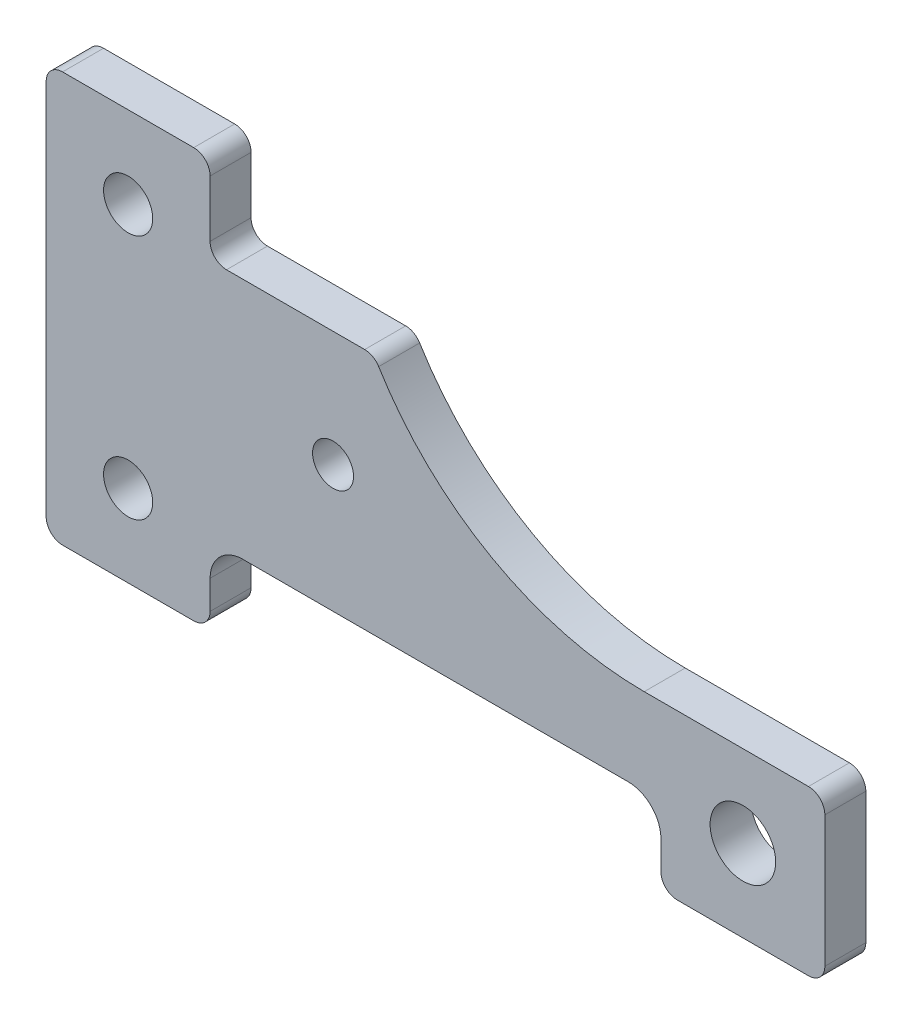
ISO-10303-21;
HEADER;
FILE_DESCRIPTION(('STEP AP214'),'2;1');
FILE_NAME('part.step','',(''),(''),'','','');
FILE_SCHEMA(('AUTOMOTIVE_DESIGN { 1 0 10303 214 1 1 1 1 }'));
ENDSEC;
DATA;
#1=APPLICATION_CONTEXT('core data for automotive mechanical design processes');
#2=APPLICATION_PROTOCOL_DEFINITION('international standard','automotive_design',2000,#1);
#3=PRODUCT_CONTEXT('',#1,'mechanical');
#4=PRODUCT('Part','Part','',(#3));
#5=PRODUCT_RELATED_PRODUCT_CATEGORY('part','',(#4));
#6=PRODUCT_DEFINITION_FORMATION('','',#4);
#7=PRODUCT_DEFINITION_CONTEXT('part definition',#1,'design');
#8=PRODUCT_DEFINITION('design','',#6,#7);
#9=PRODUCT_DEFINITION_SHAPE('','',#8);
#10=(LENGTH_UNIT() NAMED_UNIT(*) SI_UNIT(.MILLI.,.METRE.));
#11=(NAMED_UNIT(*) PLANE_ANGLE_UNIT() SI_UNIT($,.RADIAN.));
#12=(NAMED_UNIT(*) SI_UNIT($,.STERADIAN.) SOLID_ANGLE_UNIT());
#13=UNCERTAINTY_MEASURE_WITH_UNIT(LENGTH_MEASURE(1.E-05),#10,'distance_accuracy_value','');
#14=(GEOMETRIC_REPRESENTATION_CONTEXT(3) GLOBAL_UNCERTAINTY_ASSIGNED_CONTEXT((#13)) GLOBAL_UNIT_ASSIGNED_CONTEXT((#10,
#11,#12)) REPRESENTATION_CONTEXT('',''));
#15=CARTESIAN_POINT('',(0.,0.,0.));
#16=DIRECTION('',(0.,0.,1.));
#17=DIRECTION('',(1.,0.,0.));
#18=AXIS2_PLACEMENT_3D('',#15,#16,#17);
#19=CARTESIAN_POINT('',(336.307967431103,311.308411214953,25.));
#20=DIRECTION('',(0.,0.,-1.));
#21=DIRECTION('',(-1.,0.,0.));
#22=AXIS2_PLACEMENT_3D('',#19,#20,#21);
#23=PLANE('',#22);
#24=CARTESIAN_POINT('',(336.307967431103,311.308411214953,25.));
#25=DIRECTION('',(0.,0.,-1.));
#26=DIRECTION('',(-1.,0.,0.));
#27=AXIS2_PLACEMENT_3D('',#24,#25,#26);
#28=CIRCLE('',#27,380.);
#29=CARTESIAN_POINT('',(336.307967431103,-68.6915887850467,25.));
#30=VERTEX_POINT('',#29);
#31=CARTESIAN_POINT('',(12.3249909625088,112.725856697819,25.));
#32=VERTEX_POINT('',#31);
#33=EDGE_CURVE('E271',#30,#32,#28,.T.);
#34=ORIENTED_EDGE('',*,*,#33,.T.);
#35=CARTESIAN_POINT('',(-4.72674464110145,102.274143302181,25.));
#36=DIRECTION('',(0.,0.,1.));
#37=DIRECTION('',(-1.,0.,0.));
#38=AXIS2_PLACEMENT_3D('',#35,#36,#37);
#39=CIRCLE('',#38,20.);
#40=CARTESIAN_POINT('',(-4.72674464110145,122.274143302181,25.));
#41=VERTEX_POINT('',#40);
#42=EDGE_CURVE('E145',#32,#41,#39,.T.);
#43=ORIENTED_EDGE('',*,*,#42,.T.);
#44=DIRECTION('',(-1.,0.,0.));
#45=VECTOR('',#44,1.);
#46=CARTESIAN_POINT('',(-173.337365547664,122.274143302181,25.));
#47=LINE('',#46,#45);
#48=CARTESIAN_POINT('',(-173.337365547664,122.274143302181,25.));
#49=VERTEX_POINT('',#48);
#50=EDGE_CURVE('E332',#41,#49,#47,.T.);
#51=ORIENTED_EDGE('',*,*,#50,.T.);
#52=CARTESIAN_POINT('',(-173.337365547664,142.274143302181,25.));
#53=DIRECTION('',(0.,0.,-1.));
#54=DIRECTION('',(1.,0.,0.));
#55=AXIS2_PLACEMENT_3D('',#52,#53,#54);
#56=CIRCLE('',#55,20.);
#57=CARTESIAN_POINT('',(-193.337365547664,142.274143302181,25.));
#58=VERTEX_POINT('',#57);
#59=EDGE_CURVE('E348',#49,#58,#56,.T.);
#60=ORIENTED_EDGE('',*,*,#59,.T.);
#61=DIRECTION('',(0.,1.,0.));
#62=VECTOR('',#61,1.);
#63=CARTESIAN_POINT('',(-193.337365547664,211.308411214953,25.));
#64=LINE('',#63,#62);
#65=CARTESIAN_POINT('',(-193.337365547664,211.308411214953,25.));
#66=VERTEX_POINT('',#65);
#67=EDGE_CURVE('E350',#58,#66,#64,.T.);
#68=ORIENTED_EDGE('',*,*,#67,.T.);
#69=CARTESIAN_POINT('',(-213.337365547664,211.308411214953,25.));
#70=DIRECTION('',(0.,0.,1.));
#71=DIRECTION('',(1.,0.,0.));
#72=AXIS2_PLACEMENT_3D('',#69,#70,#71);
#73=CIRCLE('',#72,20.);
#74=CARTESIAN_POINT('',(-213.337365547664,231.308411214953,25.));
#75=VERTEX_POINT('',#74);
#76=EDGE_CURVE('E349',#66,#75,#73,.T.);
#77=ORIENTED_EDGE('',*,*,#76,.T.);
#78=DIRECTION('',(-1.,0.,0.));
#79=VECTOR('',#78,1.);
#80=CARTESIAN_POINT('',(-373.337365547664,231.308411214953,25.));
#81=LINE('',#80,#79);
#82=CARTESIAN_POINT('',(-373.337365547664,231.308411214953,25.));
#83=VERTEX_POINT('',#82);
#84=EDGE_CURVE('E355',#75,#83,#81,.T.);
#85=ORIENTED_EDGE('',*,*,#84,.T.);
#86=CARTESIAN_POINT('',(-373.337365547664,211.308411214953,25.));
#87=DIRECTION('',(0.,0.,1.));
#88=DIRECTION('',(-1.,0.,0.));
#89=AXIS2_PLACEMENT_3D('',#86,#87,#88);
#90=CIRCLE('',#89,20.);
#91=CARTESIAN_POINT('',(-393.337365547664,211.308411214953,25.));
#92=VERTEX_POINT('',#91);
#93=EDGE_CURVE('E360',#83,#92,#90,.T.);
#94=ORIENTED_EDGE('',*,*,#93,.T.);
#95=DIRECTION('',(0.,-1.,0.));
#96=VECTOR('',#95,1.);
#97=CARTESIAN_POINT('',(-393.337365547664,211.308411214953,25.));
#98=LINE('',#97,#96);
#99=CARTESIAN_POINT('',(-393.337365547664,-248.691588785047,25.));
#100=VERTEX_POINT('',#99);
#101=EDGE_CURVE('E357',#92,#100,#98,.T.);
#102=ORIENTED_EDGE('',*,*,#101,.T.);
#103=CARTESIAN_POINT('',(-373.337365547664,-248.691588785047,25.));
#104=DIRECTION('',(0.,0.,1.));
#105=DIRECTION('',(1.,0.,0.));
#106=AXIS2_PLACEMENT_3D('',#103,#104,#105);
#107=CIRCLE('',#106,20.);
#108=CARTESIAN_POINT('',(-373.337365547664,-268.691588785047,25.));
#109=VERTEX_POINT('',#108);
#110=EDGE_CURVE('E362',#100,#109,#107,.T.);
#111=ORIENTED_EDGE('',*,*,#110,.T.);
#112=DIRECTION('',(1.,0.,0.));
#113=VECTOR('',#112,1.);
#114=CARTESIAN_POINT('',(-373.337365547664,-268.691588785047,25.));
#115=LINE('',#114,#113);
#116=CARTESIAN_POINT('',(-213.337365547664,-268.691588785047,25.));
#117=VERTEX_POINT('',#116);
#118=EDGE_CURVE('E365',#109,#117,#115,.T.);
#119=ORIENTED_EDGE('',*,*,#118,.T.);
#120=CARTESIAN_POINT('',(-213.337365547664,-248.691588785047,25.));
#121=DIRECTION('',(0.,0.,1.));
#122=DIRECTION('',(1.,0.,0.));
#123=AXIS2_PLACEMENT_3D('',#120,#121,#122);
#124=CIRCLE('',#123,20.);
#125=CARTESIAN_POINT('',(-193.337365547664,-248.691588785047,25.));
#126=VERTEX_POINT('',#125);
#127=EDGE_CURVE('E368',#117,#126,#124,.T.);
#128=ORIENTED_EDGE('',*,*,#127,.T.);
#129=DIRECTION('',(0.,1.,0.));
#130=VECTOR('',#129,1.);
#131=CARTESIAN_POINT('',(-193.337365547664,-248.691588785047,25.));
#132=LINE('',#131,#130);
#133=CARTESIAN_POINT('',(-193.337365547664,-213.676012461059,25.));
#134=VERTEX_POINT('',#133);
#135=EDGE_CURVE('E366',#126,#134,#132,.T.);
#136=ORIENTED_EDGE('',*,*,#135,.T.);
#137=CARTESIAN_POINT('',(-153.337365547664,-213.676012461059,25.));
#138=DIRECTION('',(0.,0.,-1.));
#139=DIRECTION('',(-1.,0.,0.));
#140=AXIS2_PLACEMENT_3D('',#137,#138,#139);
#141=CIRCLE('',#140,40.);
#142=CARTESIAN_POINT('',(-153.337365547664,-173.676012461059,25.));
#143=VERTEX_POINT('',#142);
#144=EDGE_CURVE('E367',#134,#143,#141,.T.);
#145=ORIENTED_EDGE('',*,*,#144,.T.);
#146=DIRECTION('',(1.,0.,0.));
#147=VECTOR('',#146,1.);
#148=CARTESIAN_POINT('',(-153.337365547664,-173.676012461059,25.));
#149=LINE('',#148,#147);
#150=CARTESIAN_POINT('',(316.662634452336,-173.676012461059,25.));
#151=VERTEX_POINT('',#150);
#152=EDGE_CURVE('E375',#143,#151,#149,.T.);
#153=ORIENTED_EDGE('',*,*,#152,.T.);
#154=CARTESIAN_POINT('',(316.662634452336,-213.676012461059,25.));
#155=DIRECTION('',(0.,0.,-1.));
#156=DIRECTION('',(-1.,0.,0.));
#157=AXIS2_PLACEMENT_3D('',#154,#155,#156);
#158=CIRCLE('',#157,40.);
#159=CARTESIAN_POINT('',(356.662634452336,-213.676012461059,25.));
#160=VERTEX_POINT('',#159);
#161=EDGE_CURVE('E372',#151,#160,#158,.T.);
#162=ORIENTED_EDGE('',*,*,#161,.T.);
#163=DIRECTION('',(0.,-1.,0.));
#164=VECTOR('',#163,1.);
#165=CARTESIAN_POINT('',(356.662634452336,-213.676012461059,25.));
#166=LINE('',#165,#164);
#167=CARTESIAN_POINT('',(356.662634452336,-248.691588785047,25.));
#168=VERTEX_POINT('',#167);
#169=EDGE_CURVE('E376',#160,#168,#166,.T.);
#170=ORIENTED_EDGE('',*,*,#169,.T.);
#171=CARTESIAN_POINT('',(376.662634452336,-248.691588785047,25.));
#172=DIRECTION('',(0.,0.,1.));
#173=DIRECTION('',(1.,0.,0.));
#174=AXIS2_PLACEMENT_3D('',#171,#172,#173);
#175=CIRCLE('',#174,20.);
#176=CARTESIAN_POINT('',(376.662634452336,-268.691588785047,25.));
#177=VERTEX_POINT('',#176);
#178=EDGE_CURVE('E378',#168,#177,#175,.T.);
#179=ORIENTED_EDGE('',*,*,#178,.T.);
#180=DIRECTION('',(1.,0.,0.));
#181=VECTOR('',#180,1.);
#182=CARTESIAN_POINT('',(376.662634452336,-268.691588785047,25.));
#183=LINE('',#182,#181);
#184=CARTESIAN_POINT('',(536.662634452336,-268.691588785047,25.));
#185=VERTEX_POINT('',#184);
#186=EDGE_CURVE('E379',#177,#185,#183,.T.);
#187=ORIENTED_EDGE('',*,*,#186,.T.);
#188=CARTESIAN_POINT('',(536.662634452336,-248.691588785047,25.));
#189=DIRECTION('',(0.,0.,1.));
#190=DIRECTION('',(1.,0.,0.));
#191=AXIS2_PLACEMENT_3D('',#188,#189,#190);
#192=CIRCLE('',#191,20.);
#193=CARTESIAN_POINT('',(556.662634452336,-248.691588785047,25.));
#194=VERTEX_POINT('',#193);
#195=EDGE_CURVE('E208',#185,#194,#192,.T.);
#196=ORIENTED_EDGE('',*,*,#195,.T.);
#197=DIRECTION('',(0.,1.,0.));
#198=VECTOR('',#197,1.);
#199=CARTESIAN_POINT('',(556.662634452336,-248.691588785047,25.));
#200=LINE('',#199,#198);
#201=CARTESIAN_POINT('',(556.662634452336,-88.6915887850468,25.));
#202=VERTEX_POINT('',#201);
#203=EDGE_CURVE('E205',#194,#202,#200,.T.);
#204=ORIENTED_EDGE('',*,*,#203,.T.);
#205=CARTESIAN_POINT('',(536.662634452336,-88.6915887850467,25.));
#206=DIRECTION('',(0.,0.,1.));
#207=DIRECTION('',(1.,0.,0.));
#208=AXIS2_PLACEMENT_3D('',#205,#206,#207);
#209=CIRCLE('',#208,20.);
#210=CARTESIAN_POINT('',(536.662634452336,-68.6915887850467,25.));
#211=VERTEX_POINT('',#210);
#212=EDGE_CURVE('E206',#202,#211,#209,.T.);
#213=ORIENTED_EDGE('',*,*,#212,.T.);
#214=DIRECTION('',(-1.,0.,0.));
#215=VECTOR('',#214,1.);
#216=CARTESIAN_POINT('',(536.662634452336,-68.6915887850467,25.));
#217=LINE('',#216,#215);
#218=EDGE_CURVE('E57',#211,#30,#217,.T.);
#219=ORIENTED_EDGE('',*,*,#218,.T.);
#220=EDGE_LOOP('',(#34,#43,#51,#60,#68,#77,#85,#94,#102,#111,#119,#128,#136,#145,#153,#162,#170,
#179,#187,#196,#204,#213,#219));
#221=FACE_BOUND('',#220,.T.);
#222=CARTESIAN_POINT('',(-293.337365547664,131.308411214953,25.));
#223=DIRECTION('',(0.,0.,1.));
#224=DIRECTION('',(1.,0.,0.));
#225=AXIS2_PLACEMENT_3D('',#222,#223,#224);
#226=CIRCLE('',#225,30.);
#227=CARTESIAN_POINT('',(-263.337365547664,131.308411214953,25.));
#228=VERTEX_POINT('',#227);
#229=EDGE_CURVE('E229',#228,#228,#226,.T.);
#230=ORIENTED_EDGE('',*,*,#229,.F.);
#231=EDGE_LOOP('',(#230));
#232=FACE_BOUND('',#231,.T.);
#233=CARTESIAN_POINT('',(-293.337365547664,-168.691588785047,25.));
#234=DIRECTION('',(0.,0.,1.));
#235=DIRECTION('',(1.,0.,0.));
#236=AXIS2_PLACEMENT_3D('',#233,#234,#235);
#237=CIRCLE('',#236,30.);
#238=CARTESIAN_POINT('',(-263.337365547664,-168.691588785047,25.));
#239=VERTEX_POINT('',#238);
#240=EDGE_CURVE('E441',#239,#239,#237,.T.);
#241=ORIENTED_EDGE('',*,*,#240,.F.);
#242=EDGE_LOOP('',(#241));
#243=FACE_BOUND('',#242,.T.);
#244=CARTESIAN_POINT('',(-43.337365547664,-18.6915887850467,25.));
#245=DIRECTION('',(0.,0.,1.));
#246=DIRECTION('',(1.,0.,0.));
#247=AXIS2_PLACEMENT_3D('',#244,#245,#246);
#248=CIRCLE('',#247,25.);
#249=CARTESIAN_POINT('',(-18.337365547664,-18.6915887850467,25.));
#250=VERTEX_POINT('',#249);
#251=EDGE_CURVE('E437',#250,#250,#248,.T.);
#252=ORIENTED_EDGE('',*,*,#251,.F.);
#253=EDGE_LOOP('',(#252));
#254=FACE_BOUND('',#253,.T.);
#255=CARTESIAN_POINT('',(456.662634452336,-168.691588785047,25.));
#256=DIRECTION('',(0.,0.,1.));
#257=DIRECTION('',(1.,0.,0.));
#258=AXIS2_PLACEMENT_3D('',#255,#256,#257);
#259=CIRCLE('',#258,40.);
#260=CARTESIAN_POINT('',(496.662634452336,-168.691588785047,25.));
#261=VERTEX_POINT('',#260);
#262=EDGE_CURVE('E427',#261,#261,#259,.T.);
#263=ORIENTED_EDGE('',*,*,#262,.F.);
#264=EDGE_LOOP('',(#263));
#265=FACE_BOUND('',#264,.T.);
#266=ADVANCED_FACE('F39',(#221,#232,#243,#254,#265),#23,.F.);
#267=CARTESIAN_POINT('',(336.307967431103,311.308411214953,-25.));
#268=DIRECTION('',(0.,0.,-1.));
#269=DIRECTION('',(-1.,0.,0.));
#270=AXIS2_PLACEMENT_3D('',#267,#268,#269);
#271=PLANE('',#270);
#272=CARTESIAN_POINT('',(-43.337365547664,-18.6915887850467,-25.));
#273=DIRECTION('',(0.,0.,1.));
#274=DIRECTION('',(1.,0.,0.));
#275=AXIS2_PLACEMENT_3D('',#272,#273,#274);
#276=CIRCLE('',#275,25.);
#277=CARTESIAN_POINT('',(-18.337365547664,-18.6915887850467,-25.));
#278=VERTEX_POINT('',#277);
#279=EDGE_CURVE('E434',#278,#278,#276,.T.);
#280=ORIENTED_EDGE('',*,*,#279,.T.);
#281=EDGE_LOOP('',(#280));
#282=FACE_BOUND('',#281,.T.);
#283=CARTESIAN_POINT('',(-293.337365547664,131.308411214953,-25.));
#284=DIRECTION('',(0.,0.,1.));
#285=DIRECTION('',(1.,0.,0.));
#286=AXIS2_PLACEMENT_3D('',#283,#284,#285);
#287=CIRCLE('',#286,30.);
#288=CARTESIAN_POINT('',(-263.337365547664,131.308411214953,-25.));
#289=VERTEX_POINT('',#288);
#290=EDGE_CURVE('E450',#289,#289,#287,.T.);
#291=ORIENTED_EDGE('',*,*,#290,.T.);
#292=EDGE_LOOP('',(#291));
#293=FACE_BOUND('',#292,.T.);
#294=CARTESIAN_POINT('',(336.307967431103,311.308411214953,-25.));
#295=DIRECTION('',(0.,0.,-1.));
#296=DIRECTION('',(-1.,0.,0.));
#297=AXIS2_PLACEMENT_3D('',#294,#295,#296);
#298=CIRCLE('',#297,380.);
#299=CARTESIAN_POINT('',(336.307967431103,-68.6915887850467,-25.));
#300=VERTEX_POINT('',#299);
#301=CARTESIAN_POINT('',(12.3249909625088,112.725856697819,-25.));
#302=VERTEX_POINT('',#301);
#303=EDGE_CURVE('E226',#300,#302,#298,.T.);
#304=ORIENTED_EDGE('',*,*,#303,.F.);
#305=DIRECTION('',(-1.,0.,0.));
#306=VECTOR('',#305,1.);
#307=CARTESIAN_POINT('',(536.662634452336,-68.6915887850467,-25.));
#308=LINE('',#307,#306);
#309=CARTESIAN_POINT('',(536.662634452336,-68.6915887850467,-25.));
#310=VERTEX_POINT('',#309);
#311=EDGE_CURVE('E139',#310,#300,#308,.T.);
#312=ORIENTED_EDGE('',*,*,#311,.F.);
#313=CARTESIAN_POINT('',(536.662634452336,-88.6915887850467,-25.));
#314=DIRECTION('',(0.,0.,1.));
#315=DIRECTION('',(1.,0.,0.));
#316=AXIS2_PLACEMENT_3D('',#313,#314,#315);
#317=CIRCLE('',#316,20.);
#318=CARTESIAN_POINT('',(556.662634452336,-88.6915887850468,-25.));
#319=VERTEX_POINT('',#318);
#320=EDGE_CURVE('E128',#319,#310,#317,.T.);
#321=ORIENTED_EDGE('',*,*,#320,.F.);
#322=DIRECTION('',(0.,1.,0.));
#323=VECTOR('',#322,1.);
#324=CARTESIAN_POINT('',(556.662634452336,-248.691588785047,-25.));
#325=LINE('',#324,#323);
#326=CARTESIAN_POINT('',(556.662634452336,-248.691588785047,-25.));
#327=VERTEX_POINT('',#326);
#328=EDGE_CURVE('E216',#327,#319,#325,.T.);
#329=ORIENTED_EDGE('',*,*,#328,.F.);
#330=CARTESIAN_POINT('',(536.662634452336,-248.691588785047,-25.));
#331=DIRECTION('',(0.,0.,1.));
#332=DIRECTION('',(1.,0.,0.));
#333=AXIS2_PLACEMENT_3D('',#330,#331,#332);
#334=CIRCLE('',#333,20.);
#335=CARTESIAN_POINT('',(536.662634452336,-268.691588785047,-25.));
#336=VERTEX_POINT('',#335);
#337=EDGE_CURVE('E266',#336,#327,#334,.T.);
#338=ORIENTED_EDGE('',*,*,#337,.F.);
#339=DIRECTION('',(1.,0.,0.));
#340=VECTOR('',#339,1.);
#341=CARTESIAN_POINT('',(376.662634452336,-268.691588785047,-25.));
#342=LINE('',#341,#340);
#343=CARTESIAN_POINT('',(376.662634452336,-268.691588785047,-25.));
#344=VERTEX_POINT('',#343);
#345=EDGE_CURVE('E262',#344,#336,#342,.T.);
#346=ORIENTED_EDGE('',*,*,#345,.F.);
#347=CARTESIAN_POINT('',(376.662634452336,-248.691588785047,-25.));
#348=DIRECTION('',(0.,0.,1.));
#349=DIRECTION('',(1.,0.,0.));
#350=AXIS2_PLACEMENT_3D('',#347,#348,#349);
#351=CIRCLE('',#350,20.);
#352=CARTESIAN_POINT('',(356.662634452336,-248.691588785047,-25.));
#353=VERTEX_POINT('',#352);
#354=EDGE_CURVE('E265',#353,#344,#351,.T.);
#355=ORIENTED_EDGE('',*,*,#354,.F.);
#356=DIRECTION('',(0.,-1.,0.));
#357=VECTOR('',#356,1.);
#358=CARTESIAN_POINT('',(356.662634452336,-213.676012461059,-25.));
#359=LINE('',#358,#357);
#360=CARTESIAN_POINT('',(356.662634452336,-213.676012461059,-25.));
#361=VERTEX_POINT('',#360);
#362=EDGE_CURVE('E257',#361,#353,#359,.T.);
#363=ORIENTED_EDGE('',*,*,#362,.F.);
#364=CARTESIAN_POINT('',(316.662634452336,-213.676012461059,-25.));
#365=DIRECTION('',(0.,0.,-1.));
#366=DIRECTION('',(-1.,0.,0.));
#367=AXIS2_PLACEMENT_3D('',#364,#365,#366);
#368=CIRCLE('',#367,40.);
#369=CARTESIAN_POINT('',(316.662634452336,-173.676012461059,-25.));
#370=VERTEX_POINT('',#369);
#371=EDGE_CURVE('E256',#370,#361,#368,.T.);
#372=ORIENTED_EDGE('',*,*,#371,.F.);
#373=DIRECTION('',(1.,0.,0.));
#374=VECTOR('',#373,1.);
#375=CARTESIAN_POINT('',(-153.337365547664,-173.676012461059,-25.));
#376=LINE('',#375,#374);
#377=CARTESIAN_POINT('',(-153.337365547664,-173.676012461059,-25.));
#378=VERTEX_POINT('',#377);
#379=EDGE_CURVE('E258',#378,#370,#376,.T.);
#380=ORIENTED_EDGE('',*,*,#379,.F.);
#381=CARTESIAN_POINT('',(-153.337365547664,-213.676012461059,-25.));
#382=DIRECTION('',(0.,0.,-1.));
#383=DIRECTION('',(-1.,0.,0.));
#384=AXIS2_PLACEMENT_3D('',#381,#382,#383);
#385=CIRCLE('',#384,40.);
#386=CARTESIAN_POINT('',(-193.337365547664,-213.676012461059,-25.));
#387=VERTEX_POINT('',#386);
#388=EDGE_CURVE('E255',#387,#378,#385,.T.);
#389=ORIENTED_EDGE('',*,*,#388,.F.);
#390=DIRECTION('',(0.,1.,0.));
#391=VECTOR('',#390,1.);
#392=CARTESIAN_POINT('',(-193.337365547664,-248.691588785047,-25.));
#393=LINE('',#392,#391);
#394=CARTESIAN_POINT('',(-193.337365547664,-248.691588785047,-25.));
#395=VERTEX_POINT('',#394);
#396=EDGE_CURVE('E252',#395,#387,#393,.T.);
#397=ORIENTED_EDGE('',*,*,#396,.F.);
#398=CARTESIAN_POINT('',(-213.337365547664,-248.691588785047,-25.));
#399=DIRECTION('',(0.,0.,1.));
#400=DIRECTION('',(1.,0.,0.));
#401=AXIS2_PLACEMENT_3D('',#398,#399,#400);
#402=CIRCLE('',#401,20.);
#403=CARTESIAN_POINT('',(-213.337365547664,-268.691588785047,-25.));
#404=VERTEX_POINT('',#403);
#405=EDGE_CURVE('E247',#404,#395,#402,.T.);
#406=ORIENTED_EDGE('',*,*,#405,.F.);
#407=DIRECTION('',(1.,0.,0.));
#408=VECTOR('',#407,1.);
#409=CARTESIAN_POINT('',(-373.337365547664,-268.691588785047,-25.));
#410=LINE('',#409,#408);
#411=CARTESIAN_POINT('',(-373.337365547664,-268.691588785047,-25.));
#412=VERTEX_POINT('',#411);
#413=EDGE_CURVE('E250',#412,#404,#410,.T.);
#414=ORIENTED_EDGE('',*,*,#413,.F.);
#415=CARTESIAN_POINT('',(-373.337365547664,-248.691588785047,-25.));
#416=DIRECTION('',(0.,0.,1.));
#417=DIRECTION('',(1.,0.,0.));
#418=AXIS2_PLACEMENT_3D('',#415,#416,#417);
#419=CIRCLE('',#418,20.);
#420=CARTESIAN_POINT('',(-393.337365547664,-248.691588785047,-25.));
#421=VERTEX_POINT('',#420);
#422=EDGE_CURVE('E249',#421,#412,#419,.T.);
#423=ORIENTED_EDGE('',*,*,#422,.F.);
#424=DIRECTION('',(0.,-1.,0.));
#425=VECTOR('',#424,1.);
#426=CARTESIAN_POINT('',(-393.337365547664,211.308411214953,-25.));
#427=LINE('',#426,#425);
#428=CARTESIAN_POINT('',(-393.337365547664,211.308411214953,-25.));
#429=VERTEX_POINT('',#428);
#430=EDGE_CURVE('E243',#429,#421,#427,.T.);
#431=ORIENTED_EDGE('',*,*,#430,.F.);
#432=CARTESIAN_POINT('',(-373.337365547664,211.308411214953,-25.));
#433=DIRECTION('',(0.,0.,1.));
#434=DIRECTION('',(-1.,0.,0.));
#435=AXIS2_PLACEMENT_3D('',#432,#433,#434);
#436=CIRCLE('',#435,20.);
#437=CARTESIAN_POINT('',(-373.337365547664,231.308411214953,-25.));
#438=VERTEX_POINT('',#437);
#439=EDGE_CURVE('E245',#438,#429,#436,.T.);
#440=ORIENTED_EDGE('',*,*,#439,.F.);
#441=DIRECTION('',(-1.,0.,0.));
#442=VECTOR('',#441,1.);
#443=CARTESIAN_POINT('',(-373.337365547664,231.308411214953,-25.));
#444=LINE('',#443,#442);
#445=CARTESIAN_POINT('',(-213.337365547664,231.308411214953,-25.));
#446=VERTEX_POINT('',#445);
#447=EDGE_CURVE('E238',#446,#438,#444,.T.);
#448=ORIENTED_EDGE('',*,*,#447,.F.);
#449=CARTESIAN_POINT('',(-213.337365547664,211.308411214953,-25.));
#450=DIRECTION('',(0.,0.,1.));
#451=DIRECTION('',(1.,0.,0.));
#452=AXIS2_PLACEMENT_3D('',#449,#450,#451);
#453=CIRCLE('',#452,20.);
#454=CARTESIAN_POINT('',(-193.337365547664,211.308411214953,-25.));
#455=VERTEX_POINT('',#454);
#456=EDGE_CURVE('E236',#455,#446,#453,.T.);
#457=ORIENTED_EDGE('',*,*,#456,.F.);
#458=DIRECTION('',(0.,1.,0.));
#459=VECTOR('',#458,1.);
#460=CARTESIAN_POINT('',(-193.337365547664,211.308411214953,-25.));
#461=LINE('',#460,#459);
#462=CARTESIAN_POINT('',(-193.337365547664,142.274143302181,-25.));
#463=VERTEX_POINT('',#462);
#464=EDGE_CURVE('E237',#463,#455,#461,.T.);
#465=ORIENTED_EDGE('',*,*,#464,.F.);
#466=CARTESIAN_POINT('',(-173.337365547664,142.274143302181,-25.));
#467=DIRECTION('',(0.,0.,-1.));
#468=DIRECTION('',(1.,0.,0.));
#469=AXIS2_PLACEMENT_3D('',#466,#467,#468);
#470=CIRCLE('',#469,20.);
#471=CARTESIAN_POINT('',(-173.337365547664,122.274143302181,-25.));
#472=VERTEX_POINT('',#471);
#473=EDGE_CURVE('E233',#472,#463,#470,.T.);
#474=ORIENTED_EDGE('',*,*,#473,.F.);
#475=DIRECTION('',(-1.,0.,0.));
#476=VECTOR('',#475,1.);
#477=CARTESIAN_POINT('',(-173.337365547664,122.274143302181,-25.));
#478=LINE('',#477,#476);
#479=CARTESIAN_POINT('',(-4.72674464110145,122.274143302181,-25.));
#480=VERTEX_POINT('',#479);
#481=EDGE_CURVE('E231',#480,#472,#478,.T.);
#482=ORIENTED_EDGE('',*,*,#481,.F.);
#483=CARTESIAN_POINT('',(-4.72674464110145,102.274143302181,-25.));
#484=DIRECTION('',(0.,0.,1.));
#485=DIRECTION('',(-1.,0.,0.));
#486=AXIS2_PLACEMENT_3D('',#483,#484,#485);
#487=CIRCLE('',#486,20.);
#488=EDGE_CURVE('E228',#302,#480,#487,.T.);
#489=ORIENTED_EDGE('',*,*,#488,.F.);
#490=EDGE_LOOP('',(#304,#312,#321,#329,#338,#346,#355,#363,#372,#380,#389,#397,#406,#414,#423,
#431,#440,#448,#457,#465,#474,#482,#489));
#491=FACE_BOUND('',#490,.T.);
#492=CARTESIAN_POINT('',(-293.337365547664,-168.691588785047,-25.));
#493=DIRECTION('',(0.,0.,1.));
#494=DIRECTION('',(1.,0.,0.));
#495=AXIS2_PLACEMENT_3D('',#492,#493,#494);
#496=CIRCLE('',#495,30.);
#497=CARTESIAN_POINT('',(-263.337365547664,-168.691588785047,-25.));
#498=VERTEX_POINT('',#497);
#499=EDGE_CURVE('E442',#498,#498,#496,.T.);
#500=ORIENTED_EDGE('',*,*,#499,.T.);
#501=EDGE_LOOP('',(#500));
#502=FACE_BOUND('',#501,.T.);
#503=CARTESIAN_POINT('',(456.662634452336,-168.691588785047,-25.));
#504=DIRECTION('',(0.,0.,1.));
#505=DIRECTION('',(1.,0.,0.));
#506=AXIS2_PLACEMENT_3D('',#503,#504,#505);
#507=CIRCLE('',#506,40.);
#508=CARTESIAN_POINT('',(496.662634452336,-168.691588785047,-25.));
#509=VERTEX_POINT('',#508);
#510=EDGE_CURVE('E435',#509,#509,#507,.T.);
#511=ORIENTED_EDGE('',*,*,#510,.T.);
#512=EDGE_LOOP('',(#511));
#513=FACE_BOUND('',#512,.T.);
#514=ADVANCED_FACE('F333',(#282,#293,#491,#502,#513),#271,.T.);
#515=CARTESIAN_POINT('',(336.307967431103,311.308411214953,25.));
#516=DIRECTION('',(0.,0.,-1.));
#517=DIRECTION('',(-1.,0.,0.));
#518=AXIS2_PLACEMENT_3D('',#515,#516,#517);
#519=CYLINDRICAL_SURFACE('',#518,380.);
#520=ORIENTED_EDGE('',*,*,#303,.T.);
#521=DIRECTION('',(0.,0.,-1.));
#522=VECTOR('',#521,1.);
#523=CARTESIAN_POINT('',(12.3249909625088,112.725856697819,25.));
#524=LINE('',#523,#522);
#525=EDGE_CURVE('E11',#32,#302,#524,.T.);
#526=ORIENTED_EDGE('',*,*,#525,.F.);
#527=ORIENTED_EDGE('',*,*,#33,.F.);
#528=DIRECTION('',(0.,0.,-1.));
#529=VECTOR('',#528,1.);
#530=CARTESIAN_POINT('',(336.307967431103,-68.6915887850467,25.));
#531=LINE('',#530,#529);
#532=EDGE_CURVE('E225',#30,#300,#531,.T.);
#533=ORIENTED_EDGE('',*,*,#532,.T.);
#534=EDGE_LOOP('',(#520,#526,#527,#533));
#535=FACE_BOUND('',#534,.T.);
#536=ADVANCED_FACE('F41',(#535),#519,.F.);
#537=CARTESIAN_POINT('',(-4.72674464110145,102.274143302181,25.));
#538=DIRECTION('',(0.,0.,-1.));
#539=DIRECTION('',(-1.,0.,0.));
#540=AXIS2_PLACEMENT_3D('',#537,#538,#539);
#541=CYLINDRICAL_SURFACE('',#540,20.);
#542=ORIENTED_EDGE('',*,*,#488,.T.);
#543=DIRECTION('',(0.,0.,-1.));
#544=VECTOR('',#543,1.);
#545=CARTESIAN_POINT('',(-4.72674464110145,122.274143302181,25.));
#546=LINE('',#545,#544);
#547=EDGE_CURVE('E48',#41,#480,#546,.T.);
#548=ORIENTED_EDGE('',*,*,#547,.F.);
#549=ORIENTED_EDGE('',*,*,#42,.F.);
#550=ORIENTED_EDGE('',*,*,#525,.T.);
#551=EDGE_LOOP('',(#542,#548,#549,#550));
#552=FACE_BOUND('',#551,.T.);
#553=ADVANCED_FACE('F675',(#552),#541,.T.);
#554=CARTESIAN_POINT('',(-173.337365547664,122.274143302181,25.));
#555=DIRECTION('',(0.,-1.,0.));
#556=DIRECTION('',(0.,0.,-1.));
#557=AXIS2_PLACEMENT_3D('',#554,#555,#556);
#558=PLANE('',#557);
#559=ORIENTED_EDGE('',*,*,#481,.T.);
#560=DIRECTION('',(0.,0.,-1.));
#561=VECTOR('',#560,1.);
#562=CARTESIAN_POINT('',(-173.337365547664,122.274143302181,25.));
#563=LINE('',#562,#561);
#564=EDGE_CURVE('E323',#49,#472,#563,.T.);
#565=ORIENTED_EDGE('',*,*,#564,.F.);
#566=ORIENTED_EDGE('',*,*,#50,.F.);
#567=ORIENTED_EDGE('',*,*,#547,.T.);
#568=EDGE_LOOP('',(#559,#565,#566,#567));
#569=FACE_BOUND('',#568,.T.);
#570=ADVANCED_FACE('F328',(#569),#558,.F.);
#571=CARTESIAN_POINT('',(-173.337365547664,142.274143302181,25.));
#572=DIRECTION('',(0.,0.,-1.));
#573=DIRECTION('',(-1.,0.,0.));
#574=AXIS2_PLACEMENT_3D('',#571,#572,#573);
#575=CYLINDRICAL_SURFACE('',#574,20.);
#576=ORIENTED_EDGE('',*,*,#473,.T.);
#577=DIRECTION('',(0.,0.,-1.));
#578=VECTOR('',#577,1.);
#579=CARTESIAN_POINT('',(-193.337365547664,142.274143302181,25.));
#580=LINE('',#579,#578);
#581=EDGE_CURVE('E319',#58,#463,#580,.T.);
#582=ORIENTED_EDGE('',*,*,#581,.F.);
#583=ORIENTED_EDGE('',*,*,#59,.F.);
#584=ORIENTED_EDGE('',*,*,#564,.T.);
#585=EDGE_LOOP('',(#576,#582,#583,#584));
#586=FACE_BOUND('',#585,.T.);
#587=ADVANCED_FACE('F344',(#586),#575,.F.);
#588=CARTESIAN_POINT('',(-193.337365547664,211.308411214953,25.));
#589=DIRECTION('',(-1.,0.,0.));
#590=DIRECTION('',(0.,0.,1.));
#591=AXIS2_PLACEMENT_3D('',#588,#589,#590);
#592=PLANE('',#591);
#593=ORIENTED_EDGE('',*,*,#464,.T.);
#594=DIRECTION('',(0.,0.,-1.));
#595=VECTOR('',#594,1.);
#596=CARTESIAN_POINT('',(-193.337365547664,211.308411214953,25.));
#597=LINE('',#596,#595);
#598=EDGE_CURVE('E320',#66,#455,#597,.T.);
#599=ORIENTED_EDGE('',*,*,#598,.F.);
#600=ORIENTED_EDGE('',*,*,#67,.F.);
#601=ORIENTED_EDGE('',*,*,#581,.T.);
#602=EDGE_LOOP('',(#593,#599,#600,#601));
#603=FACE_BOUND('',#602,.T.);
#604=ADVANCED_FACE('F342',(#603),#592,.F.);
#605=CARTESIAN_POINT('',(-213.337365547664,211.308411214953,25.));
#606=DIRECTION('',(0.,0.,-1.));
#607=DIRECTION('',(-1.,0.,0.));
#608=AXIS2_PLACEMENT_3D('',#605,#606,#607);
#609=CYLINDRICAL_SURFACE('',#608,20.);
#610=ORIENTED_EDGE('',*,*,#456,.T.);
#611=DIRECTION('',(0.,0.,-1.));
#612=VECTOR('',#611,1.);
#613=CARTESIAN_POINT('',(-213.337365547664,231.308411214953,25.));
#614=LINE('',#613,#612);
#615=EDGE_CURVE('E314',#75,#446,#614,.T.);
#616=ORIENTED_EDGE('',*,*,#615,.F.);
#617=ORIENTED_EDGE('',*,*,#76,.F.);
#618=ORIENTED_EDGE('',*,*,#598,.T.);
#619=EDGE_LOOP('',(#610,#616,#617,#618));
#620=FACE_BOUND('',#619,.T.);
#621=ADVANCED_FACE('F636',(#620),#609,.T.);
#622=CARTESIAN_POINT('',(-373.337365547664,231.308411214953,25.));
#623=DIRECTION('',(0.,-1.,0.));
#624=DIRECTION('',(1.,0.,0.));
#625=AXIS2_PLACEMENT_3D('',#622,#623,#624);
#626=PLANE('',#625);
#627=ORIENTED_EDGE('',*,*,#447,.T.);
#628=DIRECTION('',(0.,0.,-1.));
#629=VECTOR('',#628,1.);
#630=CARTESIAN_POINT('',(-373.337365547664,231.308411214953,25.));
#631=LINE('',#630,#629);
#632=EDGE_CURVE('E313',#83,#438,#631,.T.);
#633=ORIENTED_EDGE('',*,*,#632,.F.);
#634=ORIENTED_EDGE('',*,*,#84,.F.);
#635=ORIENTED_EDGE('',*,*,#615,.T.);
#636=EDGE_LOOP('',(#627,#633,#634,#635));
#637=FACE_BOUND('',#636,.T.);
#638=ADVANCED_FACE('F627',(#637),#626,.F.);
#639=CARTESIAN_POINT('',(-373.337365547664,211.308411214953,25.));
#640=DIRECTION('',(0.,0.,-1.));
#641=DIRECTION('',(-1.,0.,0.));
#642=AXIS2_PLACEMENT_3D('',#639,#640,#641);
#643=CYLINDRICAL_SURFACE('',#642,20.);
#644=ORIENTED_EDGE('',*,*,#439,.T.);
#645=DIRECTION('',(0.,0.,-1.));
#646=VECTOR('',#645,1.);
#647=CARTESIAN_POINT('',(-393.337365547664,211.308411214953,25.));
#648=LINE('',#647,#646);
#649=EDGE_CURVE('E306',#92,#429,#648,.T.);
#650=ORIENTED_EDGE('',*,*,#649,.F.);
#651=ORIENTED_EDGE('',*,*,#93,.F.);
#652=ORIENTED_EDGE('',*,*,#632,.T.);
#653=EDGE_LOOP('',(#644,#650,#651,#652));
#654=FACE_BOUND('',#653,.T.);
#655=ADVANCED_FACE('F620',(#654),#643,.T.);
#656=CARTESIAN_POINT('',(-393.337365547664,211.308411214953,25.));
#657=DIRECTION('',(1.,0.,0.));
#658=DIRECTION('',(0.,0.,-1.));
#659=AXIS2_PLACEMENT_3D('',#656,#657,#658);
#660=PLANE('',#659);
#661=ORIENTED_EDGE('',*,*,#430,.T.);
#662=DIRECTION('',(0.,0.,-1.));
#663=VECTOR('',#662,1.);
#664=CARTESIAN_POINT('',(-393.337365547664,-248.691588785047,25.));
#665=LINE('',#664,#663);
#666=EDGE_CURVE('E302',#100,#421,#665,.T.);
#667=ORIENTED_EDGE('',*,*,#666,.F.);
#668=ORIENTED_EDGE('',*,*,#101,.F.);
#669=ORIENTED_EDGE('',*,*,#649,.T.);
#670=EDGE_LOOP('',(#661,#667,#668,#669));
#671=FACE_BOUND('',#670,.T.);
#672=ADVANCED_FACE('F609',(#671),#660,.F.);
#673=CARTESIAN_POINT('',(-373.337365547664,-248.691588785047,25.));
#674=DIRECTION('',(0.,0.,-1.));
#675=DIRECTION('',(-1.,0.,0.));
#676=AXIS2_PLACEMENT_3D('',#673,#674,#675);
#677=CYLINDRICAL_SURFACE('',#676,20.);
#678=ORIENTED_EDGE('',*,*,#422,.T.);
#679=DIRECTION('',(0.,0.,-1.));
#680=VECTOR('',#679,1.);
#681=CARTESIAN_POINT('',(-373.337365547664,-268.691588785047,25.));
#682=LINE('',#681,#680);
#683=EDGE_CURVE('E301',#109,#412,#682,.T.);
#684=ORIENTED_EDGE('',*,*,#683,.F.);
#685=ORIENTED_EDGE('',*,*,#110,.F.);
#686=ORIENTED_EDGE('',*,*,#666,.T.);
#687=EDGE_LOOP('',(#678,#684,#685,#686));
#688=FACE_BOUND('',#687,.T.);
#689=ADVANCED_FACE('F598',(#688),#677,.T.);
#690=CARTESIAN_POINT('',(-373.337365547664,-268.691588785047,25.));
#691=DIRECTION('',(0.,1.,0.));
#692=DIRECTION('',(0.,0.,1.));
#693=AXIS2_PLACEMENT_3D('',#690,#691,#692);
#694=PLANE('',#693);
#695=ORIENTED_EDGE('',*,*,#413,.T.);
#696=DIRECTION('',(0.,0.,-1.));
#697=VECTOR('',#696,1.);
#698=CARTESIAN_POINT('',(-213.337365547664,-268.691588785047,25.));
#699=LINE('',#698,#697);
#700=EDGE_CURVE('E298',#117,#404,#699,.T.);
#701=ORIENTED_EDGE('',*,*,#700,.F.);
#702=ORIENTED_EDGE('',*,*,#118,.F.);
#703=ORIENTED_EDGE('',*,*,#683,.T.);
#704=EDGE_LOOP('',(#695,#701,#702,#703));
#705=FACE_BOUND('',#704,.T.);
#706=ADVANCED_FACE('F586',(#705),#694,.F.);
#707=CARTESIAN_POINT('',(-213.337365547664,-248.691588785047,25.));
#708=DIRECTION('',(0.,0.,-1.));
#709=DIRECTION('',(-1.,0.,0.));
#710=AXIS2_PLACEMENT_3D('',#707,#708,#709);
#711=CYLINDRICAL_SURFACE('',#710,20.);
#712=ORIENTED_EDGE('',*,*,#405,.T.);
#713=DIRECTION('',(0.,0.,-1.));
#714=VECTOR('',#713,1.);
#715=CARTESIAN_POINT('',(-193.337365547664,-248.691588785047,25.));
#716=LINE('',#715,#714);
#717=EDGE_CURVE('E296',#126,#395,#716,.T.);
#718=ORIENTED_EDGE('',*,*,#717,.F.);
#719=ORIENTED_EDGE('',*,*,#127,.F.);
#720=ORIENTED_EDGE('',*,*,#700,.T.);
#721=EDGE_LOOP('',(#712,#718,#719,#720));
#722=FACE_BOUND('',#721,.T.);
#723=ADVANCED_FACE('F580',(#722),#711,.T.);
#724=CARTESIAN_POINT('',(-193.337365547664,-248.691588785047,25.));
#725=DIRECTION('',(-1.,0.,0.));
#726=DIRECTION('',(0.,0.,1.));
#727=AXIS2_PLACEMENT_3D('',#724,#725,#726);
#728=PLANE('',#727);
#729=ORIENTED_EDGE('',*,*,#396,.T.);
#730=DIRECTION('',(0.,0.,-1.));
#731=VECTOR('',#730,1.);
#732=CARTESIAN_POINT('',(-193.337365547664,-213.676012461059,25.));
#733=LINE('',#732,#731);
#734=EDGE_CURVE('E291',#134,#387,#733,.T.);
#735=ORIENTED_EDGE('',*,*,#734,.F.);
#736=ORIENTED_EDGE('',*,*,#135,.F.);
#737=ORIENTED_EDGE('',*,*,#717,.T.);
#738=EDGE_LOOP('',(#729,#735,#736,#737));
#739=FACE_BOUND('',#738,.T.);
#740=ADVANCED_FACE('F566',(#739),#728,.F.);
#741=CARTESIAN_POINT('',(-153.337365547664,-213.676012461059,25.));
#742=DIRECTION('',(0.,0.,-1.));
#743=DIRECTION('',(-1.,0.,0.));
#744=AXIS2_PLACEMENT_3D('',#741,#742,#743);
#745=CYLINDRICAL_SURFACE('',#744,40.);
#746=ORIENTED_EDGE('',*,*,#388,.T.);
#747=DIRECTION('',(0.,0.,-1.));
#748=VECTOR('',#747,1.);
#749=CARTESIAN_POINT('',(-153.337365547664,-173.676012461059,25.));
#750=LINE('',#749,#748);
#751=EDGE_CURVE('E287',#143,#378,#750,.T.);
#752=ORIENTED_EDGE('',*,*,#751,.F.);
#753=ORIENTED_EDGE('',*,*,#144,.F.);
#754=ORIENTED_EDGE('',*,*,#734,.T.);
#755=EDGE_LOOP('',(#746,#752,#753,#754));
#756=FACE_BOUND('',#755,.T.);
#757=ADVANCED_FACE('F557',(#756),#745,.F.);
#758=CARTESIAN_POINT('',(-153.337365547664,-173.676012461059,25.));
#759=DIRECTION('',(0.,1.,0.));
#760=DIRECTION('',(0.,0.,1.));
#761=AXIS2_PLACEMENT_3D('',#758,#759,#760);
#762=PLANE('',#761);
#763=ORIENTED_EDGE('',*,*,#379,.T.);
#764=DIRECTION('',(0.,0.,-1.));
#765=VECTOR('',#764,1.);
#766=CARTESIAN_POINT('',(316.662634452336,-173.676012461059,25.));
#767=LINE('',#766,#765);
#768=EDGE_CURVE('E286',#151,#370,#767,.T.);
#769=ORIENTED_EDGE('',*,*,#768,.F.);
#770=ORIENTED_EDGE('',*,*,#152,.F.);
#771=ORIENTED_EDGE('',*,*,#751,.T.);
#772=EDGE_LOOP('',(#763,#769,#770,#771));
#773=FACE_BOUND('',#772,.T.);
#774=ADVANCED_FACE('F547',(#773),#762,.F.);
#775=CARTESIAN_POINT('',(316.662634452336,-213.676012461059,25.));
#776=DIRECTION('',(0.,0.,-1.));
#777=DIRECTION('',(-1.,0.,0.));
#778=AXIS2_PLACEMENT_3D('',#775,#776,#777);
#779=CYLINDRICAL_SURFACE('',#778,40.);
#780=ORIENTED_EDGE('',*,*,#371,.T.);
#781=DIRECTION('',(0.,0.,-1.));
#782=VECTOR('',#781,1.);
#783=CARTESIAN_POINT('',(356.662634452336,-213.676012461059,25.));
#784=LINE('',#783,#782);
#785=EDGE_CURVE('E283',#160,#361,#784,.T.);
#786=ORIENTED_EDGE('',*,*,#785,.F.);
#787=ORIENTED_EDGE('',*,*,#161,.F.);
#788=ORIENTED_EDGE('',*,*,#768,.T.);
#789=EDGE_LOOP('',(#780,#786,#787,#788));
#790=FACE_BOUND('',#789,.T.);
#791=ADVANCED_FACE('F538',(#790),#779,.F.);
#792=CARTESIAN_POINT('',(356.662634452336,-213.676012461059,25.));
#793=DIRECTION('',(1.,0.,0.));
#794=DIRECTION('',(0.,1.,0.));
#795=AXIS2_PLACEMENT_3D('',#792,#793,#794);
#796=PLANE('',#795);
#797=ORIENTED_EDGE('',*,*,#362,.T.);
#798=DIRECTION('',(0.,0.,-1.));
#799=VECTOR('',#798,1.);
#800=CARTESIAN_POINT('',(356.662634452336,-248.691588785047,25.));
#801=LINE('',#800,#799);
#802=EDGE_CURVE('E281',#168,#353,#801,.T.);
#803=ORIENTED_EDGE('',*,*,#802,.F.);
#804=ORIENTED_EDGE('',*,*,#169,.F.);
#805=ORIENTED_EDGE('',*,*,#785,.T.);
#806=EDGE_LOOP('',(#797,#803,#804,#805));
#807=FACE_BOUND('',#806,.T.);
#808=ADVANCED_FACE('F526',(#807),#796,.F.);
#809=CARTESIAN_POINT('',(376.662634452336,-248.691588785047,25.));
#810=DIRECTION('',(0.,0.,-1.));
#811=DIRECTION('',(-1.,0.,0.));
#812=AXIS2_PLACEMENT_3D('',#809,#810,#811);
#813=CYLINDRICAL_SURFACE('',#812,20.);
#814=ORIENTED_EDGE('',*,*,#354,.T.);
#815=DIRECTION('',(0.,0.,-1.));
#816=VECTOR('',#815,1.);
#817=CARTESIAN_POINT('',(376.662634452336,-268.691588785047,25.));
#818=LINE('',#817,#816);
#819=EDGE_CURVE('E279',#177,#344,#818,.T.);
#820=ORIENTED_EDGE('',*,*,#819,.F.);
#821=ORIENTED_EDGE('',*,*,#178,.F.);
#822=ORIENTED_EDGE('',*,*,#802,.T.);
#823=EDGE_LOOP('',(#814,#820,#821,#822));
#824=FACE_BOUND('',#823,.T.);
#825=ADVANCED_FACE('F518',(#824),#813,.T.);
#826=CARTESIAN_POINT('',(376.662634452336,-268.691588785047,25.));
#827=DIRECTION('',(0.,1.,0.));
#828=DIRECTION('',(0.,0.,1.));
#829=AXIS2_PLACEMENT_3D('',#826,#827,#828);
#830=PLANE('',#829);
#831=ORIENTED_EDGE('',*,*,#345,.T.);
#832=DIRECTION('',(0.,0.,-1.));
#833=VECTOR('',#832,1.);
#834=CARTESIAN_POINT('',(536.662634452336,-268.691588785047,25.));
#835=LINE('',#834,#833);
#836=EDGE_CURVE('E274',#185,#336,#835,.T.);
#837=ORIENTED_EDGE('',*,*,#836,.F.);
#838=ORIENTED_EDGE('',*,*,#186,.F.);
#839=ORIENTED_EDGE('',*,*,#819,.T.);
#840=EDGE_LOOP('',(#831,#837,#838,#839));
#841=FACE_BOUND('',#840,.T.);
#842=ADVANCED_FACE('F387',(#841),#830,.F.);
#843=CARTESIAN_POINT('',(536.662634452336,-248.691588785047,25.));
#844=DIRECTION('',(0.,0.,-1.));
#845=DIRECTION('',(-1.,0.,0.));
#846=AXIS2_PLACEMENT_3D('',#843,#844,#845);
#847=CYLINDRICAL_SURFACE('',#846,20.);
#848=ORIENTED_EDGE('',*,*,#337,.T.);
#849=DIRECTION('',(0.,0.,-1.));
#850=VECTOR('',#849,1.);
#851=CARTESIAN_POINT('',(556.662634452336,-248.691588785047,25.));
#852=LINE('',#851,#850);
#853=EDGE_CURVE('E220',#194,#327,#852,.T.);
#854=ORIENTED_EDGE('',*,*,#853,.F.);
#855=ORIENTED_EDGE('',*,*,#195,.F.);
#856=ORIENTED_EDGE('',*,*,#836,.T.);
#857=EDGE_LOOP('',(#848,#854,#855,#856));
#858=FACE_BOUND('',#857,.T.);
#859=ADVANCED_FACE('F388',(#858),#847,.T.);
#860=CARTESIAN_POINT('',(556.662634452336,-248.691588785047,25.));
#861=DIRECTION('',(-1.,0.,0.));
#862=DIRECTION('',(0.,-1.,0.));
#863=AXIS2_PLACEMENT_3D('',#860,#861,#862);
#864=PLANE('',#863);
#865=ORIENTED_EDGE('',*,*,#328,.T.);
#866=DIRECTION('',(0.,0.,-1.));
#867=VECTOR('',#866,1.);
#868=CARTESIAN_POINT('',(556.662634452336,-88.6915887850468,25.));
#869=LINE('',#868,#867);
#870=EDGE_CURVE('E213',#202,#319,#869,.T.);
#871=ORIENTED_EDGE('',*,*,#870,.F.);
#872=ORIENTED_EDGE('',*,*,#203,.F.);
#873=ORIENTED_EDGE('',*,*,#853,.T.);
#874=EDGE_LOOP('',(#865,#871,#872,#873));
#875=FACE_BOUND('',#874,.T.);
#876=ADVANCED_FACE('F212',(#875),#864,.F.);
#877=CARTESIAN_POINT('',(536.662634452336,-88.6915887850467,25.));
#878=DIRECTION('',(0.,0.,-1.));
#879=DIRECTION('',(-1.,0.,0.));
#880=AXIS2_PLACEMENT_3D('',#877,#878,#879);
#881=CYLINDRICAL_SURFACE('',#880,20.);
#882=ORIENTED_EDGE('',*,*,#320,.T.);
#883=DIRECTION('',(0.,0.,-1.));
#884=VECTOR('',#883,1.);
#885=CARTESIAN_POINT('',(536.662634452336,-68.6915887850467,25.));
#886=LINE('',#885,#884);
#887=EDGE_CURVE('E217',#211,#310,#886,.T.);
#888=ORIENTED_EDGE('',*,*,#887,.F.);
#889=ORIENTED_EDGE('',*,*,#212,.F.);
#890=ORIENTED_EDGE('',*,*,#870,.T.);
#891=EDGE_LOOP('',(#882,#888,#889,#890));
#892=FACE_BOUND('',#891,.T.);
#893=ADVANCED_FACE('F219',(#892),#881,.T.);
#894=CARTESIAN_POINT('',(536.662634452336,-68.6915887850467,25.));
#895=DIRECTION('',(0.,-1.,0.));
#896=DIRECTION('',(0.,0.,-1.));
#897=AXIS2_PLACEMENT_3D('',#894,#895,#896);
#898=PLANE('',#897);
#899=ORIENTED_EDGE('',*,*,#311,.T.);
#900=ORIENTED_EDGE('',*,*,#532,.F.);
#901=ORIENTED_EDGE('',*,*,#218,.F.);
#902=ORIENTED_EDGE('',*,*,#887,.T.);
#903=EDGE_LOOP('',(#899,#900,#901,#902));
#904=FACE_BOUND('',#903,.T.);
#905=ADVANCED_FACE('F393',(#904),#898,.F.);
#906=CARTESIAN_POINT('',(-293.337365547664,131.308411214953,25.));
#907=DIRECTION('',(0.,0.,-1.));
#908=DIRECTION('',(-1.,0.,0.));
#909=AXIS2_PLACEMENT_3D('',#906,#907,#908);
#910=CYLINDRICAL_SURFACE('',#909,30.);
#911=ORIENTED_EDGE('',*,*,#229,.T.);
#912=EDGE_LOOP('',(#911));
#913=FACE_BOUND('',#912,.T.);
#914=ORIENTED_EDGE('',*,*,#290,.F.);
#915=EDGE_LOOP('',(#914));
#916=FACE_BOUND('',#915,.T.);
#917=ADVANCED_FACE('F399',(#913,#916),#910,.F.);
#918=CARTESIAN_POINT('',(-293.337365547664,-168.691588785047,25.));
#919=DIRECTION('',(0.,0.,-1.));
#920=DIRECTION('',(-1.,0.,0.));
#921=AXIS2_PLACEMENT_3D('',#918,#919,#920);
#922=CYLINDRICAL_SURFACE('',#921,30.);
#923=ORIENTED_EDGE('',*,*,#240,.T.);
#924=EDGE_LOOP('',(#923));
#925=FACE_BOUND('',#924,.T.);
#926=ORIENTED_EDGE('',*,*,#499,.F.);
#927=EDGE_LOOP('',(#926));
#928=FACE_BOUND('',#927,.T.);
#929=ADVANCED_FACE('F405',(#925,#928),#922,.F.);
#930=CARTESIAN_POINT('',(-43.337365547664,-18.6915887850467,25.));
#931=DIRECTION('',(0.,0.,-1.));
#932=DIRECTION('',(-1.,0.,0.));
#933=AXIS2_PLACEMENT_3D('',#930,#931,#932);
#934=CYLINDRICAL_SURFACE('',#933,25.);
#935=ORIENTED_EDGE('',*,*,#251,.T.);
#936=EDGE_LOOP('',(#935));
#937=FACE_BOUND('',#936,.T.);
#938=ORIENTED_EDGE('',*,*,#279,.F.);
#939=EDGE_LOOP('',(#938));
#940=FACE_BOUND('',#939,.T.);
#941=ADVANCED_FACE('F418',(#937,#940),#934,.F.);
#942=CARTESIAN_POINT('',(456.662634452336,-168.691588785047,25.));
#943=DIRECTION('',(0.,0.,-1.));
#944=DIRECTION('',(-1.,0.,0.));
#945=AXIS2_PLACEMENT_3D('',#942,#943,#944);
#946=CYLINDRICAL_SURFACE('',#945,40.);
#947=ORIENTED_EDGE('',*,*,#262,.T.);
#948=EDGE_LOOP('',(#947));
#949=FACE_BOUND('',#948,.T.);
#950=ORIENTED_EDGE('',*,*,#510,.F.);
#951=EDGE_LOOP('',(#950));
#952=FACE_BOUND('',#951,.T.);
#953=ADVANCED_FACE('F419',(#949,#952),#946,.F.);
#954=CLOSED_SHELL('',(#266,#514,#536,#553,#570,#587,#604,#621,#638,#655,#672,#689,#706,#723,
#740,#757,#774,#791,#808,#825,#842,#859,#876,#893,#905,#917,#929,#941,#953));
#955=MANIFOLD_SOLID_BREP('B2',#954);
#956=ADVANCED_BREP_SHAPE_REPRESENTATION('',(#18,#955),#14);
#957=SHAPE_DEFINITION_REPRESENTATION(#9,#956);
ENDSEC;
END-ISO-10303-21;
